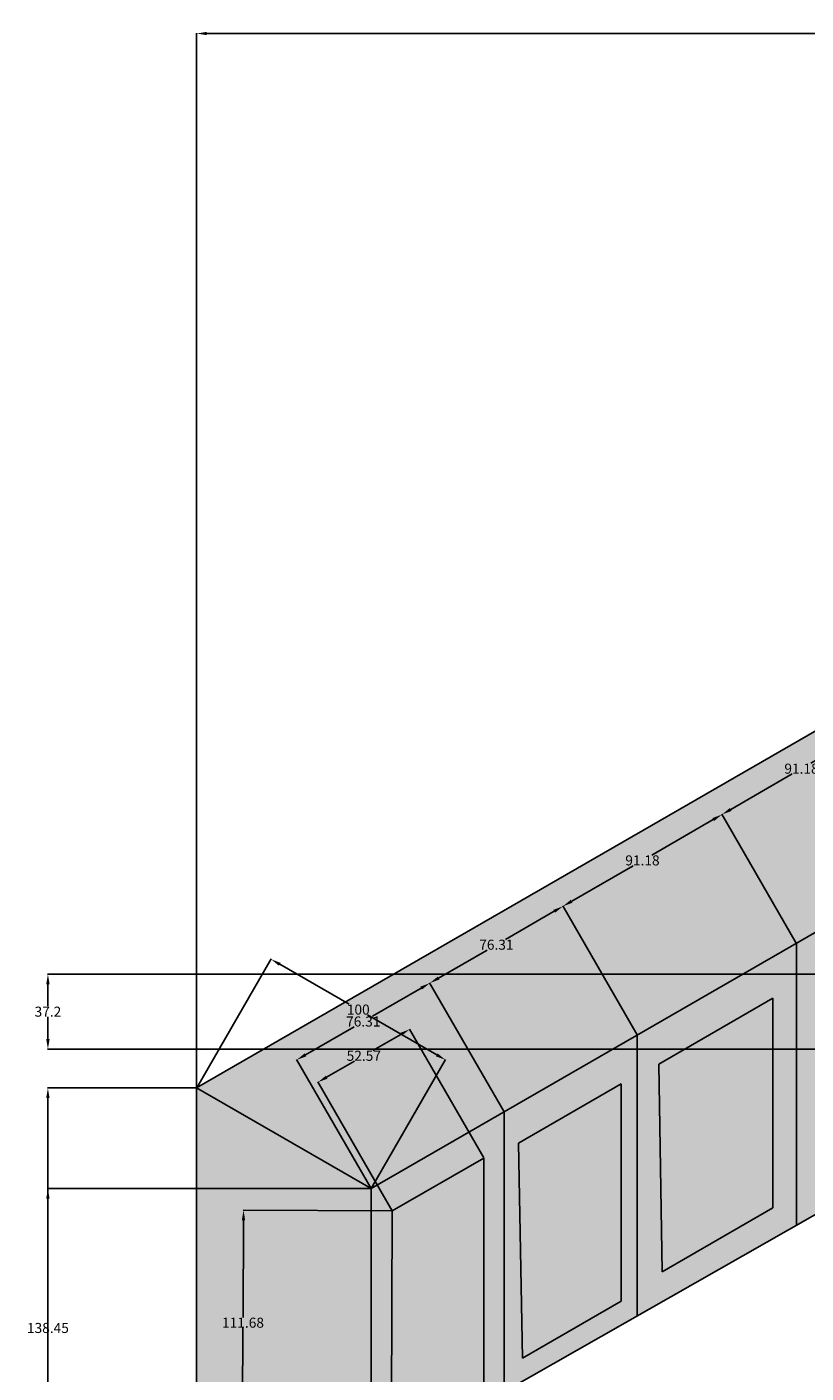
# Model space of a CAD drawing. Units: centimetres. Extents: x -744 to 1642, y 210 to 1375.
# Tile 2 of 8: x -744 to -357, y 707 to 1375. Entities that reach past the tile are written whole.
import ezdxf

# ---------------------------------------------------------------- set-up
doc = ezdxf.new("R2010")
doc.units = ezdxf.units.CM
doc.header["$MEASUREMENT"] = 0
for name, color, linetype, lineweight in [('A-ANNO-DIMS', 2, 'Continuous', 18), ('A-FURN', 7, 'Continuous', 25), ('A-FURN-PATT', 30, 'Continuous', 13), ('A-WALL-PATT', 61, 'Continuous', 13)]:
    doc.layers.add(name, color=color, linetype=linetype, lineweight=lineweight)
doc.styles.get("Standard").update_dxf_attribs({"font": 'arial.ttf'})
doc.dimstyles.get("Standard").update_dxf_attribs({"dimtxt": 5, "dimasz": 5, "dimexe": 0.18, "dimexo": 0.0625, "dimgap": 0.09, "dimtad": 0, "dimtih": 1, "dimtoh": 1, "dimdec": 0, "dimzin": 0, "dimdsep": 46, "dimtxsty": 'Standard', "dimcen": 0.09, "dimadec": 0, "dimazin": 0, "dimtfac": 1, "dimtdec": 0, "dimtofl": 0, "dimtmove": 0, "dimatfit": 3, "dimfxl": 1, "dimtolj": 1, "dimtzin": 0, "dimarcsym": 0})

# ---------------------------------------------------------------- blocks, each defined once
blk = doc.blocks.new('*D7')
at = {"layer": 'A-ANNO-DIMS', "color": 0, "lineweight": -2, "transparency": 16777216}
for p, q in [((-659.99, 848.29), (-659.99, 1372.26)), ((-654.99, 1372.08), (65.92, 1372.08)), ((807.25, 1372.08), (86.34, 1372.08)), ((812.25, 898.29), (812.25, 1372.26))]:
    blk.add_line(p, q, dxfattribs=at)
at = {"layer": 'A-ANNO-DIMS', "color": 0, "transparency": 16777216}
for points in [[(-654.99, 1372.91), (-654.99, 1371.25), (-659.99, 1372.08)], [(807.25, 1372.91), (807.25, 1371.25), (812.25, 1372.08)]]:
    blk.add_solid(points, dxfattribs=at)
at = {"layer": 'Defpoints', "color": 0, "transparency": 16777216}
for p in [(812.25, 1372.08), (812.25, 898.23), (-659.99, 848.23)]:
    blk.add_point(p, dxfattribs=at)
at = {"layer": 'A-ANNO-DIMS', "color": 0, "transparency": 16777216, "insert": (76.13, 1372.08), "char_height": 5, "attachment_point": 5}
blk.add_mtext('\\A1;1472.2', dxfattribs=at)
blk = doc.blocks.new('*D11')
at = {"layer": 'A-ANNO-DIMS', "color": 0, "lineweight": -2, "transparency": 16777216}
for p, q in [((-660.05, 848.23), (-734.02, 848.23)), ((-733.84, 843.23), (-733.84, 650.87)), ((-733.84, 453.23), (-733.84, 645.59)), ((-660.05, 448.23), (-734.02, 448.23))]:
    blk.add_line(p, q, dxfattribs=at)
at = {"layer": 'A-ANNO-DIMS', "color": 0, "transparency": 16777216}
for points in [[(-734.67, 843.23), (-733.01, 843.23), (-733.84, 848.23)], [(-734.67, 453.23), (-733.01, 453.23), (-733.84, 448.23)]]:
    blk.add_solid(points, dxfattribs=at)
at = {"layer": 'Defpoints', "color": 0, "transparency": 16777216}
for p in [(-733.84, 848.23), (-659.99, 848.23), (-659.99, 448.23)]:
    blk.add_point(p, dxfattribs=at)
at = {"layer": 'A-ANNO-DIMS', "color": 0, "transparency": 16777216, "insert": (-733.84, 648.23), "char_height": 5, "attachment_point": 5}
blk.add_mtext('\\A1;400', dxfattribs=at)
blk = doc.blocks.new('*D12')
at = {"layer": 'A-ANNO-DIMS', "color": 0, "lineweight": -2, "transparency": 16777216}
for p, q in [((-573.45, 798.23), (-734.02, 798.23)), ((-733.84, 793.23), (-733.84, 731.65)), ((-733.84, 664.78), (-733.84, 726.36)), ((-573.45, 659.78), (-734.02, 659.78))]:
    blk.add_line(p, q, dxfattribs=at)
at = {"layer": 'A-ANNO-DIMS', "color": 0, "transparency": 16777216}
for points in [[(-734.67, 793.23), (-733.01, 793.23), (-733.84, 798.23)], [(-734.67, 664.78), (-733.01, 664.78), (-733.84, 659.78)]]:
    blk.add_solid(points, dxfattribs=at)
at = {"layer": 'Defpoints', "color": 0, "transparency": 16777216}
for p in [(-573.39, 798.23), (-733.84, 659.78), (-573.39, 659.78)]:
    blk.add_point(p, dxfattribs=at)
at = {"layer": 'A-ANNO-DIMS', "color": 0, "transparency": 16777216, "insert": (-733.84, 729.01), "char_height": 5, "attachment_point": 5}
blk.add_mtext('\\A1;138.45', dxfattribs=at)
blk = doc.blocks.new('*D15')
at = {"layer": 'A-ANNO-DIMS', "color": 0, "lineweight": -2, "transparency": 16777216}
for p, q in [((-659.96, 848.28), (-622.97, 912.34)), ((-618.73, 909.69), (-584.34, 889.83)), ((-540.79, 864.69), (-575.19, 884.54)), ((-573.36, 798.28), (-536.37, 862.34))]:
    blk.add_line(p, q, dxfattribs=at)
at = {"layer": 'A-ANNO-DIMS', "color": 0, "transparency": 16777216}
for points in [[(-618.32, 910.41), (-619.15, 908.97), (-623.06, 912.19)], [(-540.38, 865.41), (-541.21, 863.97), (-536.46, 862.19)]]:
    blk.add_solid(points, dxfattribs=at)
at = {"layer": 'Defpoints', "color": 0, "transparency": 16777216}
for p in [(-536.46, 862.19), (-659.99, 848.23), (-573.39, 798.23)]:
    blk.add_point(p, dxfattribs=at)
at = {"layer": 'A-ANNO-DIMS', "color": 0, "transparency": 16777216, "insert": (-579.76, 887.19), "char_height": 5, "attachment_point": 5}
blk.add_mtext('\\A1;100', dxfattribs=at)
blk = doc.blocks.new('*D16')
at = {"layer": 'A-ANNO-DIMS', "color": 0, "lineweight": -2, "transparency": 16777216}
for p, q in [((78.18, 859.69), (-259.32, 664.83)), ((119.4, 798.28), (82.42, 862.34)), ((-605.98, 464.69), (-268.48, 659.54)), ((-573.42, 398.28), (-610.4, 462.34))]:
    blk.add_line(p, q, dxfattribs=at)
at = {"layer": 'A-ANNO-DIMS', "color": 0, "transparency": 16777216}
for points in [[(77.76, 860.41), (78.6, 858.97), (82.51, 862.19)], [(-606.4, 465.41), (-605.57, 463.97), (-610.31, 462.19)]]:
    blk.add_solid(points, dxfattribs=at)
at = {"layer": 'Defpoints', "color": 0, "transparency": 16777216}
for p in [(82.51, 862.19), (119.43, 798.23), (-573.39, 398.23)]:
    blk.add_point(p, dxfattribs=at)
at = {"layer": 'A-ANNO-DIMS', "color": 0, "transparency": 16777216, "insert": (-263.9, 662.19), "char_height": 5, "attachment_point": 5}
blk.add_mtext('\\A1;800', dxfattribs=at)
blk = doc.blocks.new('*D18')
at = {"layer": 'A-ANNO-DIMS', "color": 0, "lineweight": -2, "transparency": 16777216}
for p, q in [((-548.55, 897.84), (-572.69, 883.91)), ((-507.33, 836.44), (-544.31, 900.5)), ((-605.98, 864.69), (-581.85, 878.62)), ((-573.42, 798.28), (-610.4, 862.34))]:
    blk.add_line(p, q, dxfattribs=at)
at = {"layer": 'A-ANNO-DIMS', "color": 0, "transparency": 16777216}
for points in [[(-548.97, 898.57), (-548.14, 897.12), (-544.22, 900.34)], [(-606.4, 865.41), (-605.57, 863.97), (-610.31, 862.19)]]:
    blk.add_solid(points, dxfattribs=at)
at = {"layer": 'Defpoints', "color": 0, "transparency": 16777216}
for p in [(-544.22, 900.34), (-507.3, 836.39), (-573.39, 798.23)]:
    blk.add_point(p, dxfattribs=at)
at = {"layer": 'A-ANNO-DIMS', "color": 0, "transparency": 16777216, "insert": (-577.27, 881.27), "char_height": 5, "attachment_point": 5}
blk.add_mtext('\\A1;76.31', dxfattribs=at)
blk = doc.blocks.new('*D22')
at = {"layer": 'A-ANNO-DIMS', "color": 0, "lineweight": -2, "transparency": 16777216}
for p, q in [((-283.34, 904.75), (-734.02, 904.75)), ((-733.84, 899.75), (-733.84, 888.8)), ((-733.84, 872.55), (-733.84, 883.51)), ((-257.51, 867.55), (-734.02, 867.55))]:
    blk.add_line(p, q, dxfattribs=at)
at = {"layer": 'A-ANNO-DIMS', "color": 0, "transparency": 16777216}
for points in [[(-734.67, 899.75), (-733.01, 899.75), (-733.84, 904.75)], [(-734.67, 872.55), (-733.01, 872.55), (-733.84, 867.55)]]:
    blk.add_solid(points, dxfattribs=at)
at = {"layer": 'Defpoints', "color": 0, "transparency": 16777216}
for p in [(-283.28, 904.75), (-733.84, 867.55), (-257.44, 867.55)]:
    blk.add_point(p, dxfattribs=at)
at = {"layer": 'A-ANNO-DIMS', "color": 0, "transparency": 16777216, "insert": (-733.84, 886.15), "char_height": 5, "attachment_point": 5}
blk.add_mtext('\\A1;37.2', dxfattribs=at)
blk = doc.blocks.new('*D43')
at = {"layer": 'A-ANNO-DIMS', "color": 0, "lineweight": -2, "transparency": 16777216}
for p, q in [((-441.24, 874.6), (-478.22, 938.66)), ((-482.46, 936), (-506.6, 922.07)), ((-539.89, 902.84), (-515.76, 916.78)), ((-507.33, 836.44), (-544.31, 900.5))]:
    blk.add_line(p, q, dxfattribs=at)
at = {"layer": 'A-ANNO-DIMS', "color": 0, "transparency": 16777216}
for points in [[(-482.88, 936.72), (-482.05, 935.28), (-478.13, 938.5)], [(-540.31, 903.57), (-539.48, 902.12), (-544.22, 900.34)]]:
    blk.add_solid(points, dxfattribs=at)
at = {"layer": 'Defpoints', "color": 0, "transparency": 16777216}
for p in [(-478.13, 938.5), (-441.21, 874.54), (-507.3, 836.39)]:
    blk.add_point(p, dxfattribs=at)
at = {"layer": 'A-ANNO-DIMS', "color": 0, "transparency": 16777216, "insert": (-511.18, 919.42), "char_height": 5, "attachment_point": 5}
blk.add_mtext('\\A1;76.31', dxfattribs=at)
blk = doc.blocks.new('*D44')
at = {"layer": 'A-ANNO-DIMS', "color": 0, "lineweight": -2, "transparency": 16777216}
for p, q in [((-362.28, 920.19), (-399.26, 984.25)), ((-403.5, 981.59), (-434.07, 963.94)), ((-473.8, 941), (-443.23, 958.65)), ((-441.24, 874.6), (-478.22, 938.66))]:
    blk.add_line(p, q, dxfattribs=at)
at = {"layer": 'A-ANNO-DIMS', "color": 0, "transparency": 16777216}
for points in [[(-403.92, 982.31), (-403.08, 980.87), (-399.17, 984.09)], [(-474.22, 941.72), (-473.39, 940.28), (-478.13, 938.5)]]:
    blk.add_solid(points, dxfattribs=at)
at = {"layer": 'Defpoints', "color": 0, "transparency": 16777216}
for p in [(-399.17, 984.09), (-362.24, 920.13), (-441.21, 874.54)]:
    blk.add_point(p, dxfattribs=at)
at = {"layer": 'A-ANNO-DIMS', "color": 0, "transparency": 16777216, "insert": (-438.65, 961.3), "char_height": 5, "attachment_point": 5}
blk.add_mtext('\\A1;91.18', dxfattribs=at)
blk = doc.blocks.new('*D45')
at = {"layer": 'A-ANNO-DIMS', "color": 0, "lineweight": -2, "transparency": 16777216}
for p, q in [((-324.54, 1027.18), (-355.11, 1009.53)), ((-283.31, 965.78), (-320.3, 1029.83)), ((-394.84, 986.59), (-364.27, 1004.24)), ((-362.28, 920.19), (-399.26, 984.25))]:
    blk.add_line(p, q, dxfattribs=at)
at = {"layer": 'A-ANNO-DIMS', "color": 0, "transparency": 16777216}
for points in [[(-324.95, 1027.9), (-324.12, 1026.46), (-320.21, 1029.68)], [(-395.26, 987.31), (-394.42, 985.87), (-399.17, 984.09)]]:
    blk.add_solid(points, dxfattribs=at)
at = {"layer": 'Defpoints', "color": 0, "transparency": 16777216}
for p in [(-320.21, 1029.68), (-283.28, 965.72), (-362.24, 920.13)]:
    blk.add_point(p, dxfattribs=at)
at = {"layer": 'A-ANNO-DIMS', "color": 0, "transparency": 16777216, "insert": (-359.69, 1006.88), "char_height": 5, "attachment_point": 5}
blk.add_mtext('\\A1;91.18', dxfattribs=at)
blk = doc.blocks.new('*D64')
at = {"layer": 'A-ANNO-DIMS', "color": 0, "lineweight": -2, "transparency": 16777216}
for p, q in [((-517.36, 813.47), (-554.35, 877.53)), ((-558.59, 874.87), (-572.44, 866.87)), ((-595.46, 853.58), (-581.6, 861.58)), ((-562.89, 787.18), (-599.88, 851.24))]:
    blk.add_line(p, q, dxfattribs=at)
at = {"layer": 'A-ANNO-DIMS', "color": 0, "transparency": 16777216}
for points in [[(-559.01, 875.59), (-558.17, 874.15), (-554.26, 877.37)], [(-595.87, 854.31), (-595.04, 852.86), (-599.79, 851.08)]]:
    blk.add_solid(points, dxfattribs=at)
at = {"layer": 'Defpoints', "color": 0, "transparency": 16777216}
for p in [(-554.26, 877.37), (-517.33, 813.41), (-562.86, 787.13)]:
    blk.add_point(p, dxfattribs=at)
at = {"layer": 'A-ANNO-DIMS', "color": 0, "transparency": 16777216, "insert": (-577.02, 864.23), "char_height": 5, "attachment_point": 5}
blk.add_mtext('\\A1;52.57', dxfattribs=at)
blk = doc.blocks.new('*D65')
at = {"layer": 'A-ANNO-DIMS', "color": 0, "lineweight": -2, "transparency": 16777216}
for p, q in [((-636.73, 782.48), (-636.96, 734.29)), ((-562.92, 787.13), (-636.89, 787.48)), ((-637.22, 680.8), (-636.99, 729)), ((-563.46, 675.45), (-637.42, 675.8))]:
    blk.add_line(p, q, dxfattribs=at)
at = {"layer": 'A-ANNO-DIMS', "color": 0, "transparency": 16777216}
for points in [[(-637.57, 782.49), (-635.9, 782.48), (-636.71, 787.48)], [(-638.05, 680.81), (-636.39, 680.8), (-637.24, 675.8)]]:
    blk.add_solid(points, dxfattribs=at)
at = {"layer": 'Defpoints', "color": 0, "transparency": 16777216}
for p in [(-636.71, 787.48), (-562.86, 787.13), (-563.4, 675.45)]:
    blk.add_point(p, dxfattribs=at)
at = {"layer": 'A-ANNO-DIMS', "color": 0, "transparency": 16777216, "insert": (-636.98, 731.64), "char_height": 5, "attachment_point": 5}
blk.add_mtext('\\A1;111.68', dxfattribs=at)

msp = doc.modelspace()

# ---------------------------------------------------------------- hatches: boundary and pattern name
at = {"layer": 'A-FURN-PATT'}
h = msp.add_hatch(color=256, dxfattribs=at)
h.dxf.hatch_style = 1
h.paths.add_polyline_path([(709.906, 763.421), (709.906, 833.5619), (614.425, 888.6879), (614.425, 818.5469)])
h.paths.add_polyline_path([(482.0889, 965.0922), (482.0889, 894.9512), (580.3491, 838.2207), (580.3491, 908.3616)])
h.paths.add_polyline_path([(455.661, 989.3482), (391.7403, 1026.2528), (391.7403, 905.908), (455.661, 869.0034)])
h.paths.add_polyline_path([(367.6025, 1038.9798), (305.4698, 1074.8522), (305.4698, 959.5913), (367.6025, 923.719)])
h.paths.add_polyline_path([(283.2252, 1090.8212), (213.1748, 1130.1519), (213.1748, 1010.3029), (283.2252, 969.8593)])
h.paths.add_polyline_path([(197.085, 1142.1995), (128.5906, 1179.2565), (128.5906, 1060.1567), (197.085, 1020.6114)])
h.paths.add_polyline_path([(111.6616, 1060.697), (111.6616, 1182.612), (67.1993, 1156.9417), (67.1993, 1033.9561)])
h.paths.add_polyline_path([(51.1364, 1025.5999), (51.1364, 1146.3882), (8.133, 1121.5602), (10.63, 1002.2135)])
h.paths.add_polyline_path([(-7.1228, 994.0363), (-7.1228, 1112.7639), (-46.1416, 1090.2363), (-45.0502, 972.1389)])
h.paths.add_polyline_path([(-62.5525, 1080.1953), (-112.7586, 1051.2088), (-111.3243, 975.2962), (-98.1787, 959.5025), (-98.1787, 953.5165), (-110.7754, 946.2438), (-110.5757, 935.6761), (-62.5525, 963.4023)])
h.paths.add_polyline_path([(-131.9167, 1043.3731), (-194.3022, 1007.3548), (-194.3022, 960.6093), (-131.9167, 994.0283)])
h.paths.add_polyline_path([(-210.3768, 1001.0803), (-272.1227, 965.4313), (-272.1227, 916.524), (-210.3442, 952.1919)])
h.paths.add_polyline_path([(-295.3923, 940.164), (-352.6194, 907.1238), (-352.6194, 798.1578), (-299.691, 828.716), (-295.3923, 831.1979)])
h.paths.add_polyline_path([(-373.8641, 892.8311), (-430.554, 860.1012), (-428.9419, 756.8396), (-373.8641, 788.6388)])
h.paths.add_polyline_path([(-449.1461, 850.3626), (-500.1893, 820.8928), (-498.1887, 714.0073), (-449.1461, 742.322)])
h.paths.add_polyline_path([(-517.3336, 813.4139), (-562.861, 787.1286), (-563.3952, 675.4493), (-517.3336, 702.043)])
h.paths.add_polyline_path([(-518.4603, 570.0519), (-562.9383, 544.3726), (-563.4408, 418.3375), (-518.4603, 444.307)])
h.paths.add_polyline_path([(-371.5223, 654.8866), (-429.2034, 621.5845), (-429.2034, 495.8395), (-371.5223, 529.1417)])
h.paths.add_polyline_path([(-448.7547, 610.2965), (-500.7971, 580.2498), (-501.5895, 454.0473), (-449.5067, 484.1173)])
h.paths.add_polyline_path([(-351.4436, 666.4791), (-351.4436, 540.7341), (-295.2328, 573.1874), (-295.2328, 698.9324)])
h.paths.add_polyline_path([(-256.6887, 595.4409), (-256.6887, 687.4813), (-215.6652, 711.1662), (-215.6652, 744.8707), (-268.9239, 714.1219), (-268.9239, 588.3769)])
h.paths.add_polyline_path([(-193.7313, 723.8298), (-132.6965, 759.0682), (-132.6965, 792.7727), (-193.7313, 757.5343)])
h.paths.add_polyline_path([(-114.2, 769.7472), (-83.4836, 787.4813), (-73.2438, 781.5694), (-73.2438, 827.0978), (-114.2, 803.4517)])
h.paths.add_polyline_path([(-53.2271, 770.0128), (-7.0224, 743.3364), (-7.0224, 865.3308), (-53.2271, 838.6544)])
h.paths.add_polyline_path([(8.89, 748.7728), (52.5303, 773.9686), (52.5303, 899.7135), (8.89, 874.5177)])
h.paths.add_polyline_path([(68.067, 782.9387), (108.041, 806.0177), (108.041, 931.7626), (68.067, 908.6836)])
h.paths.add_polyline_path([(130.3442, 802.4419), (196.727, 764.1157), (196.727, 896.2228), (130.3442, 934.5489), (130.3442, 927.6391)])
h.paths.add_polyline_path([(220.7637, 875.3463), (220.7637, 755.5756), (282.3763, 720.0036), (282.3763, 835.7573), (282.3763, 840.4873)])
h.paths.add_polyline_path([(307.3754, 826.3434), (307.3754, 705.693), (368.1078, 670.6291), (368.1078, 790.9456)])
h.paths.add_polyline_path([(389.5829, 779.9795), (389.5829, 656.983), (453.252, 620.2237), (453.252, 747.8082)])
at = {"layer": 'A-WALL-PATT'}
h = msp.add_hatch(color=256, dxfattribs=at)
h.dxf.hatch_style = 1
h.paths.add_polyline_path([(-226.9766, 998.2308), (119.4335, 1198.2308), (292.6386, 1098.2308), (465.8437, 998.2308), (552.4462, 948.2308), (725.6513, 848.2308), (812.2538, 898.2308), (119.4335, 1298.2308), (-659.9893, 848.2308), (-573.3868, 798.2308)])
h.paths.add_polyline_path([(-573.3868, 798.2308), (-659.9893, 848.2308), (-659.9893, 448.2308), (-573.3868, 398.2308)])
h.paths.add_polyline_path([(-507.2972, 836.3877), (-573.3868, 798.2308), (-573.3868, 659.7809), (-507.2972, 697.4412)])
h.paths.add_polyline_path([(-562.861, 787.1286), (-517.3336, 813.4139), (-517.3336, 702.043), (-563.3952, 675.4493)], flags=16)
h.paths.add_polyline_path([(-441.2075, 735.1015), (-441.2075, 874.5446), (-507.2972, 836.3877), (-507.2972, 697.4412)])
h.paths.add_polyline_path([(-500.1893, 820.8928), (-449.1461, 850.3626), (-449.1461, 742.322), (-498.1887, 714.0073)], flags=16)
h.paths.add_polyline_path([(-362.2449, 780.0973), (-362.2449, 920.1337), (-441.2075, 874.5446), (-441.2075, 735.1015)])
h.paths.add_polyline_path([(-430.554, 860.1012), (-373.8641, 892.8311), (-373.8641, 788.6388), (-428.9419, 756.8396)], flags=16)
h.paths.add_polyline_path([(-283.2822, 825.0931), (-283.2822, 965.7228), (-362.2449, 920.1337), (-362.2449, 780.0973)])
h.paths.add_polyline_path([(-352.6194, 798.1578), (-352.6194, 907.1238), (-295.3923, 940.164), (-295.3923, 831.1979), (-299.691, 828.716)], flags=16)
h.paths.add_polyline_path([(-203.882, 947.929), (-203.5655, 1011.7473), (-226.9766, 998.2308), (-283.2822, 965.7228), (-283.2822, 904.7538)], flags=17)
h.paths.add_polyline_path([(-272.1227, 965.4313), (-210.3768, 1001.0803), (-210.3442, 952.1919), (-272.1227, 916.524)], flags=16)
h.paths.add_polyline_path([(-123.8488, 991.4483), (-123.8488, 1057.7717), (-203.5655, 1011.7473), (-203.882, 947.929)], flags=17)
h.paths.add_polyline_path([(-194.3022, 1007.3548), (-131.9167, 1043.3731), (-131.9167, 994.0283), (-194.3022, 960.6093)], flags=16)
h.paths.add_polyline_path([(-112.7586, 1051.2088), (-62.5525, 1080.1953), (-62.5525, 963.4023), (-110.5757, 935.6761), (-110.7754, 946.2438), (-123.8488, 938.6959), (-123.8488, 915.9442), (-53.7716, 955.8768), (-53.7716, 1098.2308), (-123.8488, 1057.7717), (-123.8488, 991.4483), (-123.8488, 990.3436), (-111.3243, 975.2962)], flags=17)
h.paths.add_polyline_path([(1.2011, 1129.9693), (-53.7716, 1098.2308), (-53.7716, 955.8768), (1.4435, 987.3403)], flags=17)
h.paths.add_polyline_path([(-46.1416, 1090.2363), (-7.1228, 1112.7639), (-7.1228, 994.0363), (-45.0502, 972.1389)], flags=16)
h.paths.add_polyline_path([(60.3173, 1164.1001), (1.2011, 1129.9693), (1.4435, 987.3403), (60.3173, 1020.8888)], flags=17)
h.paths.add_polyline_path([(8.133, 1121.5602), (51.1364, 1146.3882), (51.1364, 1025.5999), (10.63, 1002.2135)], flags=16)
h.paths.add_polyline_path([(119.4335, 1054.5754), (119.4335, 1198.2308), (60.3173, 1164.1001), (60.3173, 1020.8888)], flags=17)
h.paths.add_polyline_path([(67.1993, 1156.9417), (111.6616, 1182.612), (111.6616, 1060.697), (67.1993, 1033.9561)], flags=16)
h.paths.add_polyline_path([(206.0361, 1148.2308), (119.4335, 1198.2308), (119.4335, 1054.5754), (206.0361, 1003.7675)], flags=17)
h.paths.add_polyline_path([(128.5906, 1179.2565), (197.085, 1142.1995), (197.085, 1020.6114), (128.5906, 1060.1567)], flags=16)
h.paths.add_polyline_path([(206.0361, 1148.2308), (206.0361, 1003.7675), (292.6386, 952.9596), (292.6386, 1098.2308)], flags=17)
h.paths.add_polyline_path([(213.1748, 1130.1519), (283.2252, 1090.8212), (283.2252, 969.8593), (213.1748, 1010.3029)], flags=16)
h.paths.add_polyline_path([(292.6386, 1098.2308), (292.6386, 952.9596), (378.4066, 902.6412), (379.2411, 1048.2308)], flags=17)
h.paths.add_polyline_path([(305.4698, 1074.8522), (367.6025, 1038.9798), (367.6025, 923.719), (305.4698, 959.5913)], flags=16)
h.paths.add_polyline_path([(379.2411, 1048.2308), (378.4066, 902.6412), (465.8437, 851.3437), (465.8437, 998.2308)], flags=17)
h.paths.add_polyline_path([(391.7403, 1026.2528), (455.661, 989.3482), (455.661, 869.0034), (391.7403, 905.908)], flags=16)
h.paths.add_polyline_path([(552.4462, 948.2308), (465.8437, 998.2308), (465.8437, 891.6699), (595.7475, 816.0455), (595.7475, 923.2308)], flags=17)
h.paths.add_polyline_path([(482.0889, 965.0922), (580.3491, 908.3616), (580.3491, 838.2207), (482.0889, 894.9512)], flags=16)
h.paths.add_polyline_path([(595.7475, 923.2308), (595.7475, 816.0455), (725.6513, 740.4211), (725.6513, 848.2308)])
h.paths.add_polyline_path([(614.425, 888.6879), (709.906, 833.5619), (709.906, 763.421), (614.425, 818.5469)], flags=16)
h.paths.add_polyline_path([(812.2538, 898.2308), (725.6513, 848.2308), (725.6513, 740.4211), (725.6513, 448.2308), (812.2538, 498.2308)])
h.paths.add_polyline_path([(465.8437, 757.085), (377.8609, 807.4399), (376.9558, 649.5503), (465.8437, 598.2308)])
h.paths.add_polyline_path([(389.5829, 779.9795), (453.252, 747.8082), (453.252, 620.2237), (389.5829, 656.983)], flags=16)
h.paths.add_polyline_path([(377.8609, 807.4399), (292.6386, 856.215), (292.6386, 698.2308), (376.9558, 649.5503)])
h.paths.add_polyline_path([(368.1078, 670.6291), (307.3754, 705.693), (307.3754, 826.3434), (368.1078, 790.9456)], flags=16)
h.paths.add_polyline_path([(292.6386, 856.215), (206.0361, 905.7799), (206.0361, 748.2308), (292.6386, 698.2308)])
h.paths.add_polyline_path([(282.3763, 720.0036), (220.7637, 755.5756), (220.7637, 875.3463), (282.3763, 840.4873), (282.3763, 835.7573)], flags=16)
h.paths.add_polyline_path([(206.0361, 905.7799), (119.4335, 955.3449), (119.4335, 798.2308), (206.0361, 748.2308)])
h.paths.add_polyline_path([(196.727, 764.1157), (130.3442, 802.4419), (130.3442, 927.6391), (130.3442, 934.5489), (196.727, 896.2228)], flags=16)
h.paths.add_polyline_path([(119.4335, 955.3449), (60.5235, 921.3332), (60.5235, 764.2191), (119.4335, 798.2308)])
h.paths.add_polyline_path([(108.041, 806.0177), (68.067, 782.9387), (68.067, 908.6836), (108.041, 931.7626)], flags=16)
h.paths.add_polyline_path([(60.5235, 764.2191), (60.5235, 921.3332), (1.6135, 887.3215), (1.867, 738.2042), (3.1189, 737.4813), (8.6656, 734.279)])
h.paths.add_polyline_path([(8.89, 748.7728), (8.89, 874.5177), (52.5303, 899.7135), (52.5303, 773.9686)], flags=16)
h.paths.add_polyline_path([(1.6135, 887.3215), (-61.1176, 851.1036), (-61.1176, 774.5683), (-53.2271, 770.0128), (-53.2271, 838.6544), (-7.0224, 865.3308), (-7.0224, 743.3364), (1.867, 738.2042)])
h.paths.add_polyline_path([(-61.1176, 851.1036), (-123.8488, 814.8858), (-123.8488, 764.1765), (-114.2, 769.7472), (-114.2, 803.4517), (-73.2438, 827.0978), (-73.2438, 781.5694), (-61.1176, 774.5683)])
h.paths.add_polyline_path([(-132.6965, 792.7727), (-132.6965, 759.0682), (-123.8488, 764.1765), (-123.8488, 814.8858), (-203.5655, 768.8613), (-203.5655, 718.152), (-193.7313, 723.8298), (-193.7313, 757.5343)])
h.paths.add_polyline_path([(-203.5655, 768.8613), (-283.2822, 722.8369), (-283.2822, 565.7228), (-256.6887, 581.0766), (-256.6887, 595.4409), (-268.9239, 588.3769), (-268.9239, 714.1219), (-215.6652, 744.8707), (-215.6652, 711.1662), (-203.5655, 718.152)])
h.paths.add_polyline_path([(-283.2822, 722.8369), (-362.2449, 677.2477), (-362.2449, 520.1337), (-283.2822, 565.7228)])
h.paths.add_polyline_path([(-295.2328, 573.1874), (-351.4436, 540.7341), (-351.4436, 666.4791), (-295.2328, 698.9324)], flags=16)
h.paths.add_polyline_path([(-362.2449, 677.2477), (-441.2075, 631.6586), (-441.2075, 474.5446), (-362.2449, 520.1337)])
h.paths.add_polyline_path([(-371.5223, 529.1417), (-429.2034, 495.8395), (-429.2034, 621.5845), (-371.5223, 654.8866)], flags=16)
h.paths.add_polyline_path([(-441.2075, 631.6586), (-507.2972, 593.5018), (-507.2972, 436.3877), (-441.2075, 474.5446)])
h.paths.add_polyline_path([(-448.7547, 610.2965), (-449.5067, 484.1173), (-501.5895, 454.0473), (-500.7971, 580.2498)], flags=16)
h.paths.add_polyline_path([(-507.2972, 593.5018), (-573.3868, 555.3449), (-573.3868, 398.2308), (-507.2972, 436.3877)])
h.paths.add_polyline_path([(-518.4603, 570.0519), (-518.4603, 444.307), (-563.4408, 418.3375), (-562.9383, 544.3726)], flags=16)
h.paths.add_polyline_path([(-118.6694, 598.5582), (-123.6694, 601.445), (-123.6694, 488.0238), (-118.6694, 485.1326)], flags=17)
h.paths.add_polyline_path([(-113.6694, 595.6715), (-118.6694, 598.5582), (-118.6694, 485.1326), (-113.6694, 482.2413)], flags=17)
h.paths.add_polyline_path([(-12.0425, 536.9972), (-17.0425, 539.8839), (-17.0425, 426.3672), (-12.0425, 423.4759)], flags=17)
h.paths.add_polyline_path([(-17.0425, 539.8839), (-22.0425, 542.7707), (-22.0425, 429.2584), (-17.0425, 426.3672)], flags=17)
h.paths.add_polyline_path([(-256.6887, 687.4813), (-256.6887, 487.4813), (-248.6887, 482.8625), (-248.6887, 673.6249), (81.7215, 482.8625), (81.7215, 292.1001), (89.7215, 287.4813), (89.7215, 487.4813)])
h.paths.add_polyline_path([(-196.8604, 530.3463), (-196.7272, 512.8625), (81.7215, 352.1001), (81.7215, 369.2572)], flags=17)

# ---------------------------------------------------------------- linework, layer by layer
at = {"layer": 'A-FURN'}
for p, q in [((-659.9893, 848.2308), (119.4335, 1298.2308)), ((-226.9766, 998.2308), (-573.3868, 798.2308)), ((-362.2449, 920.1337), (-362.2449, 780.0973)), ((-430.554, 860.1012), (-373.8641, 892.8311)), ((-373.8641, 892.8311), (-373.8641, 788.6388)), ((-441.2075, 874.5446), (-441.2075, 735.1015)), ((-428.9419, 756.8396), (-430.554, 860.1012)), ((-500.1893, 820.8928), (-449.1461, 850.3626)), ((-449.1461, 850.3626), (-449.1461, 742.322)), ((-573.3868, 798.2308), (-659.9893, 848.2308)), ((-659.9893, 848.2308), (-659.9893, 448.2308)), ((-507.2972, 836.3877), (-507.2972, 697.4412)), ((-573.3868, 659.7809), (-283.2822, 825.0931)), ((-498.1887, 714.0073), (-500.1893, 820.8928)), ((-562.861, 787.1286), (-517.3336, 813.4139)), ((-517.3336, 813.4139), (-517.3336, 702.043)), ((-573.3868, 798.2308), (-573.3868, 398.2308)), ((-563.3952, 675.4493), (-562.861, 787.1286)), ((-373.8641, 788.6388), (-428.9419, 756.8396)), ((-449.1461, 742.322), (-498.1887, 714.0073))]:
    msp.add_line(p, q, dxfattribs=at)

# ---------------------------------------------------------------- dimensions: what is measured, and where the dimension line sits
at = {"layer": 'A-ANNO-DIMS'}
dim = msp.add_linear_dim(base=(812.2538, 1372.0808), p1=(-659.9893, 848.2308), p2=(812.2538, 898.2308), dimstyle='Standard', override={"dimdec": 1, "dimlfac": 1, "dimrnd": 0, "dimzin": 0, "dimdsep": 46, "dimlunit": 2}, dxfattribs=at)
dim.commit()
dim.dimension.update_dxf_attribs({"geometry": '*D7', "text_midpoint": (76.1323, 1372.0808)})
for base, p1, p2, angle, override, picture, middle in [((-320.2072, 1029.6788), (-362.2449, 920.1337), (-283.2822, 965.7228), 30, {"dimdec": 2, "dimlfac": 1, "dimrnd": 0, "dimzin": 0, "dimdsep": 46, "dimlunit": 2}, '*D45', (-359.6885, 1006.8842)), ((-399.1699, 984.0897), (-441.2075, 874.5446), (-362.2449, 920.1337), 30, {"dimdec": 2, "dimlfac": 1, "dimrnd": 0, "dimzin": 0, "dimdsep": 46, "dimlunit": 2}, '*D44', (-438.6512, 961.2951)), ((-478.1325, 938.5005), (-507.2972, 836.3877), (-441.2075, 874.5446), 30, {"dimdec": 2, "dimlfac": 1, "dimrnd": 0, "dimzin": 0, "dimdsep": 46, "dimlunit": 2}, '*D43', (-511.1773, 919.4221)), ((-536.4618, 862.1868), (-659.9893, 848.2308), (-573.3868, 798.2308), 330, {"dimdec": 0, "dimlfac": 1, "dimrnd": 0, "dimzin": 0, "dimdsep": 46, "dimlunit": 2}, '*D15', (-579.7631, 887.1868)), ((-733.8393, 867.552), (-283.2822, 904.7538), (-257.4428, 867.552), 90, {"dimdec": 1, "dimlfac": 1, "dimrnd": 0, "dimzin": 0, "dimdsep": 46, "dimlunit": 2}, '*D22', (-733.8393, 886.1529)), ((-544.2222, 900.3437), (-573.3868, 798.2308), (-507.2972, 836.3877), 30, {"dimdec": 2, "dimlfac": 1, "dimrnd": 0, "dimzin": 0, "dimdsep": 46, "dimlunit": 2}, '*D18', (-577.267, 881.2652)), ((-554.2586, 877.3699), (-562.861, 787.1286), (-517.3336, 813.4139), 30, {"dimdec": 2, "dimlfac": 1, "dimrnd": 0, "dimzin": 0, "dimdsep": 46, "dimlunit": 2}, '*D64', (-577.0223, 864.2272)), ((82.5085, 862.1868), (-573.3868, 398.2308), (119.4335, 798.2308), 30, {"dimdec": 0, "dimlfac": 1, "dimrnd": 0, "dimzin": 0, "dimdsep": 46, "dimlunit": 2}, '*D16', (-263.9016, 662.1868)), ((-733.8393, 848.2308), (-659.9893, 448.2308), (-659.9893, 848.2308), 90, {"dimdec": 0, "dimlfac": 1, "dimrnd": 0, "dimzin": 0, "dimdsep": 46, "dimlunit": 2}, '*D11', (-733.8393, 648.2308)), ((-733.8393, 659.7809), (-573.3868, 798.2308), (-573.3868, 659.7809), 90, {"dimdec": 2, "dimlfac": 1, "dimrnd": 0, "dimzin": 0, "dimdsep": 46, "dimlunit": 2}, '*D12', (-733.8393, 729.0058)), ((-636.7102, 787.4819), (-563.3952, 675.4493), (-562.861, 787.1286), 89.725961, {"dimdec": 2, "dimlfac": 1, "dimrnd": 0, "dimzin": 0, "dimdsep": 46, "dimlunit": 2}, '*D65', (-636.9772, 731.6422))]:
    dim = msp.add_linear_dim(base=base, p1=p1, p2=p2, angle=angle, dimstyle='Standard', override=override, dxfattribs=at)
    dim.commit()
    dim.dimension.update_dxf_attribs({"geometry": picture, "text_midpoint": middle})

doc.saveas('drawing.dxf')
